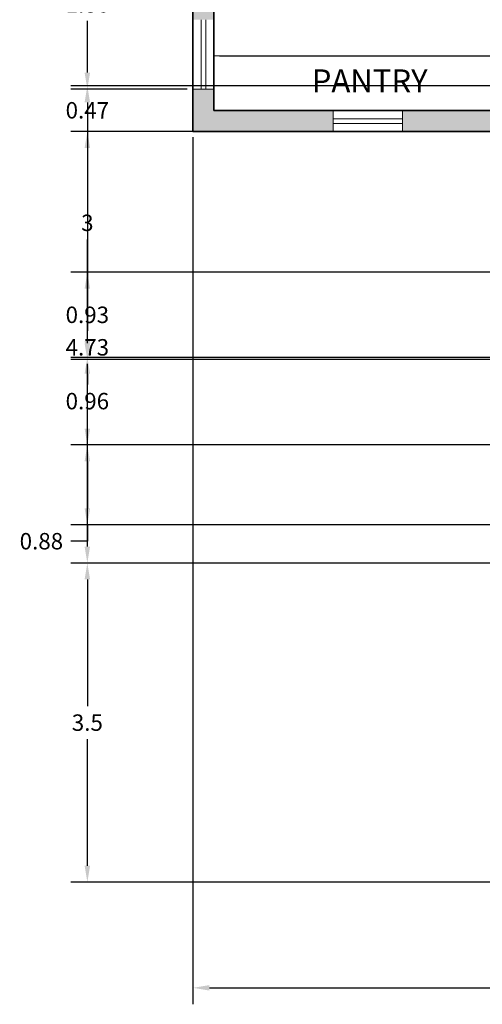
# Model space of a CAD drawing. Units: metres. Extents: x 4298.5 to 4325.2, y 2075 to 2095.8.
# Tile 1 of 35: x 4298.5 to 4303.6, y 2075 to 2085.8. Entities that reach past the tile are written whole.
import ezdxf

# ---------------------------------------------------------------- set-up
doc = ezdxf.new("R2010")
doc.units = ezdxf.units.M
for name, color, linetype, lineweight in [('A-ANNO-DIMS', 2, 'Continuous', 18), ('A-AREA-IDEN', 7, 'Continuous', 18), ('A-FLOR-CASE', 8, 'Continuous', 18), ('A-GLAZ', 4, 'Continuous', 18), ('A-WALL', 7, 'Continuous', 35), ('A-WALL-PATT', 252, 'Continuous', 13)]:
    doc.layers.add(name, color=color, linetype=linetype, lineweight=lineweight)
doc.styles.get("Standard").update_dxf_attribs({"font": 'arial.ttf'})
doc.dimstyles.get("Standard").update_dxf_attribs({"dimtxt": 0.18, "dimasz": 0.18, "dimexe": 0.18, "dimexo": 0.0625, "dimgap": 0.09, "dimtad": 0, "dimtih": 1, "dimtoh": 1, "dimdec": 4, "dimzin": 0, "dimdsep": 46, "dimtxsty": 'Standard', "dimcen": 0.09, "dimadec": 0, "dimazin": 0, "dimtfac": 1, "dimtdec": 4, "dimtofl": 0, "dimtmove": 0, "dimatfit": 3, "dimfxl": 1, "dimtolj": 1, "dimtzin": 0, "dimarcsym": 0})

# ---------------------------------------------------------------- blocks, each defined once
blk = doc.blocks.new('WIN-760-GLASS')
for p, q in [((0, 0.76), (0, 0)), ((0.05, 0.76), (0.05, 0))]:
    blk.add_line(p, q)
blk = doc.blocks.new('*D47')
at = {"layer": 'A-ANNO-DIMS', "color": 0, "lineweight": -2, "transparency": 16777216}
for p, q in [((4300.431, 2084.496), (4300.431, 2074.99)), ((4322.811, 2084.496), (4322.811, 2074.99)), ((4300.611, 2075.17), (4311.225, 2075.17)), ((4322.631, 2075.17), (4312.016, 2075.17))]:
    blk.add_line(p, q, dxfattribs=at)
at = {"layer": 'A-ANNO-DIMS', "color": 0, "transparency": 16777216}
for points in [[(4300.611, 2075.2), (4300.611, 2075.14), (4300.431, 2075.17)], [(4322.631, 2075.2), (4322.631, 2075.14), (4322.811, 2075.17)]]:
    blk.add_solid(points, dxfattribs=at)
at = {"layer": 'Defpoints', "color": 0, "transparency": 16777216}
for p in [(4300.431, 2084.558), (4322.811, 2084.558), (4322.811, 2075.17)]:
    blk.add_point(p, dxfattribs=at)
at = {"layer": 'A-ANNO-DIMS', "color": 0, "transparency": 16777216, "insert": (4311.621, 2075.17), "char_height": 0.18, "attachment_point": 5}
blk.add_mtext('\\A1;22.38', dxfattribs=at)
blk = doc.blocks.new('*D51')
at = {"layer": 'A-ANNO-DIMS', "color": 0, "lineweight": -2, "transparency": 16777216}
for p, q in [((4305.598, 2084.558), (4299.092, 2084.558)), ((4299.272, 2084.378), (4299.272, 2082.375)), ((4299.272, 2080.008), (4299.272, 2082.011)), ((4305.598, 2079.828), (4299.092, 2079.828))]:
    blk.add_line(p, q, dxfattribs=at)
at = {"layer": 'A-ANNO-DIMS', "color": 0, "transparency": 16777216}
for points in [[(4299.242, 2084.378), (4299.302, 2084.378), (4299.272, 2084.558)], [(4299.242, 2080.008), (4299.302, 2080.008), (4299.272, 2079.828)]]:
    blk.add_solid(points, dxfattribs=at)
at = {"layer": 'Defpoints', "color": 0, "transparency": 16777216}
for p in [(4305.661, 2084.558), (4299.272, 2079.828), (4305.661, 2079.828)]:
    blk.add_point(p, dxfattribs=at)
at = {"layer": 'A-ANNO-DIMS', "color": 0, "transparency": 16777216, "insert": (4299.272, 2082.193), "char_height": 0.18, "attachment_point": 5}
blk.add_mtext('\\A1;4.73', dxfattribs=at)
blk = doc.blocks.new('*D54')
at = {"layer": 'A-ANNO-DIMS', "color": 0, "lineweight": -2, "transparency": 16777216}
for p, q in [((4305.598, 2079.828), (4299.092, 2079.828)), ((4299.272, 2079.648), (4299.272, 2078.26)), ((4299.272, 2076.508), (4299.272, 2077.896)), ((4309.098, 2076.328), (4299.092, 2076.328))]:
    blk.add_line(p, q, dxfattribs=at)
at = {"layer": 'A-ANNO-DIMS', "color": 0, "transparency": 16777216}
for points in [[(4299.242, 2079.648), (4299.302, 2079.648), (4299.272, 2079.828)], [(4299.242, 2076.508), (4299.302, 2076.508), (4299.272, 2076.328)]]:
    blk.add_solid(points, dxfattribs=at)
at = {"layer": 'Defpoints', "color": 0, "transparency": 16777216}
for p in [(4305.661, 2079.828), (4299.272, 2076.328), (4309.161, 2076.328)]:
    blk.add_point(p, dxfattribs=at)
at = {"layer": 'A-ANNO-DIMS', "color": 0, "transparency": 16777216, "insert": (4299.272, 2078.078), "char_height": 0.18, "attachment_point": 5}
blk.add_mtext('\\A1;3.5', dxfattribs=at)
blk = doc.blocks.new('*D56')
at = {"layer": 'A-ANNO-DIMS', "color": 0, "lineweight": -2, "transparency": 16777216}
for p, q in [((4305.828, 2085.058), (4299.092, 2085.058)), ((4299.272, 2084.878), (4299.272, 2083.74)), ((4299.272, 2082.238), (4299.272, 2083.376)), ((4305.828, 2082.058), (4299.092, 2082.058))]:
    blk.add_line(p, q, dxfattribs=at)
at = {"layer": 'A-ANNO-DIMS', "color": 0, "transparency": 16777216}
for points in [[(4299.242, 2084.878), (4299.302, 2084.878), (4299.272, 2085.058)], [(4299.242, 2082.238), (4299.302, 2082.238), (4299.272, 2082.058)]]:
    blk.add_solid(points, dxfattribs=at)
at = {"layer": 'Defpoints', "color": 0, "transparency": 16777216}
for p in [(4299.272, 2085.058), (4305.891, 2085.058), (4305.891, 2082.058)]:
    blk.add_point(p, dxfattribs=at)
at = {"layer": 'A-ANNO-DIMS', "color": 0, "transparency": 16777216, "insert": (4299.272, 2083.558), "char_height": 0.18, "attachment_point": 5}
blk.add_mtext('\\A1;3', dxfattribs=at)
blk = doc.blocks.new('*D58')
at = {"layer": 'A-ANNO-DIMS', "color": 0, "lineweight": -2, "transparency": 16777216}
for p, q in [((4324.587, 2085.388), (4324.587, 2085.568)), ((4324.587, 2085.568), (4324.767, 2085.568)), ((4300.723, 2085.388), (4324.767, 2085.388)), ((4324.587, 2084.968), (4324.587, 2085.208)), ((4300.723, 2084.788), (4324.767, 2084.788))]:
    blk.add_line(p, q, dxfattribs=at)
at = {"layer": 'A-ANNO-DIMS', "color": 0, "transparency": 16777216}
for points in [[(4324.557, 2085.208), (4324.617, 2085.208), (4324.587, 2085.388)], [(4324.557, 2084.968), (4324.617, 2084.968), (4324.587, 2084.788)]]:
    blk.add_solid(points, dxfattribs=at)
at = {"layer": 'Defpoints', "color": 0, "transparency": 16777216}
for p in [(4300.661, 2085.388), (4324.587, 2085.388), (4300.661, 2084.788)]:
    blk.add_point(p, dxfattribs=at)
at = {"layer": 'A-ANNO-DIMS', "color": 0, "transparency": 16777216, "insert": (4325.021, 2085.568), "char_height": 0.18, "attachment_point": 5}
blk.add_mtext('\\A1;0.6', dxfattribs=at)
blk = doc.blocks.new('*D62')
at = {"layer": 'A-ANNO-DIMS', "color": 0, "lineweight": -2, "transparency": 16777216}
for p, q in [((4312.11, 2083.015), (4299.092, 2083.015)), ((4299.272, 2082.835), (4299.272, 2082.731)), ((4299.272, 2082.263), (4299.272, 2082.367)), ((4312.11, 2082.083), (4299.092, 2082.083))]:
    blk.add_line(p, q, dxfattribs=at)
at = {"layer": 'A-ANNO-DIMS', "color": 0, "transparency": 16777216}
for points in [[(4299.242, 2082.835), (4299.302, 2082.835), (4299.272, 2083.015)], [(4299.242, 2082.263), (4299.302, 2082.263), (4299.272, 2082.083)]]:
    blk.add_solid(points, dxfattribs=at)
at = {"layer": 'Defpoints', "color": 0, "transparency": 16777216}
for p in [(4312.172, 2083.015), (4299.272, 2082.083), (4312.172, 2082.083)]:
    blk.add_point(p, dxfattribs=at)
at = {"layer": 'A-ANNO-DIMS', "color": 0, "transparency": 16777216, "insert": (4299.272, 2082.549), "char_height": 0.18, "attachment_point": 5}
blk.add_mtext('\\A1;0.93', dxfattribs=at)
blk = doc.blocks.new('*D63')
at = {"layer": 'A-ANNO-DIMS', "color": 0, "lineweight": -2, "transparency": 16777216}
for p, q in [((4312.11, 2082.083), (4299.092, 2082.083)), ((4299.272, 2081.903), (4299.272, 2081.785)), ((4299.272, 2081.302), (4299.272, 2081.421)), ((4312.11, 2081.122), (4299.092, 2081.122))]:
    blk.add_line(p, q, dxfattribs=at)
at = {"layer": 'A-ANNO-DIMS', "color": 0, "transparency": 16777216}
for points in [[(4299.242, 2081.903), (4299.302, 2081.903), (4299.272, 2082.083)], [(4299.242, 2081.302), (4299.302, 2081.302), (4299.272, 2081.122)]]:
    blk.add_solid(points, dxfattribs=at)
at = {"layer": 'Defpoints', "color": 0, "transparency": 16777216}
for p in [(4312.172, 2082.083), (4299.272, 2081.122), (4312.172, 2081.122)]:
    blk.add_point(p, dxfattribs=at)
at = {"layer": 'A-ANNO-DIMS', "color": 0, "transparency": 16777216, "insert": (4299.272, 2081.603), "char_height": 0.18, "attachment_point": 5}
blk.add_mtext('\\A1;0.96', dxfattribs=at)
blk = doc.blocks.new('*D64')
at = {"layer": 'A-ANNO-DIMS', "color": 0, "lineweight": -2, "transparency": 16777216}
for p, q in [((4312.11, 2081.122), (4299.092, 2081.122)), ((4299.272, 2080.942), (4299.272, 2080.427)), ((4312.11, 2080.247), (4299.092, 2080.247)), ((4299.272, 2080.247), (4299.272, 2080.067)), ((4299.272, 2080.067), (4299.092, 2080.067))]:
    blk.add_line(p, q, dxfattribs=at)
at = {"layer": 'A-ANNO-DIMS', "color": 0, "transparency": 16777216}
for points in [[(4299.242, 2080.942), (4299.302, 2080.942), (4299.272, 2081.122)], [(4299.242, 2080.427), (4299.302, 2080.427), (4299.272, 2080.247)]]:
    blk.add_solid(points, dxfattribs=at)
at = {"layer": 'Defpoints', "color": 0, "transparency": 16777216}
for p in [(4312.172, 2081.122), (4299.272, 2080.247), (4312.172, 2080.247)]:
    blk.add_point(p, dxfattribs=at)
at = {"layer": 'A-ANNO-DIMS', "color": 0, "transparency": 16777216, "insert": (4298.768, 2080.067), "char_height": 0.18, "attachment_point": 5}
blk.add_mtext('\\A1;0.88', dxfattribs=at)
blk = doc.blocks.new('*D74')
at = {"layer": 'A-ANNO-DIMS', "color": 0, "lineweight": -2, "transparency": 16777216}
for p, q in [((4299.272077, 2085.20492), (4299.272077, 2085.38492)), ((4300.368077, 2085.02492), (4299.092077, 2085.02492)), ((4300.368077, 2084.558056), (4299.092077, 2084.558056)), ((4299.272077, 2084.378056), (4299.272077, 2084.198056))]:
    blk.add_line(p, q, dxfattribs=at)
at = {"layer": 'A-ANNO-DIMS', "color": 0, "transparency": 16777216}
for points in [[(4299.242077, 2085.20492), (4299.302077, 2085.20492), (4299.272077, 2085.02492)], [(4299.242077, 2084.378056), (4299.302077, 2084.378056), (4299.272077, 2084.558056)]]:
    blk.add_solid(points, dxfattribs=at)
at = {"layer": 'Defpoints', "color": 0, "transparency": 16777216}
for p in [(4299.272077, 2085.02492), (4300.430577, 2085.02492), (4300.430577, 2084.558056)]:
    blk.add_point(p, dxfattribs=at)
at = {"layer": 'A-ANNO-DIMS', "color": 0, "transparency": 16777216, "insert": (4299.272077, 2084.791488), "char_height": 0.18, "attachment_point": 5}
blk.add_mtext('\\A1;0.47', dxfattribs=at)
blk = doc.blocks.new('*D75')
at = {"layer": 'A-ANNO-DIMS', "color": 0, "lineweight": -2, "transparency": 16777216}
for p, q in [((4300.368, 2086.884), (4299.092, 2086.884)), ((4299.272, 2086.704), (4299.272, 2086.137)), ((4299.272, 2085.205), (4299.272, 2085.773)), ((4300.368, 2085.025), (4299.092, 2085.025))]:
    blk.add_line(p, q, dxfattribs=at)
at = {"layer": 'A-ANNO-DIMS', "color": 0, "transparency": 16777216}
for points in [[(4299.242, 2086.704), (4299.302, 2086.704), (4299.272, 2086.884)], [(4299.242, 2085.205), (4299.302, 2085.205), (4299.272, 2085.025)]]:
    blk.add_solid(points, dxfattribs=at)
at = {"layer": 'Defpoints', "color": 0, "transparency": 16777216}
for p in [(4299.272, 2086.884), (4300.431, 2086.884), (4300.431, 2085.025)]:
    blk.add_point(p, dxfattribs=at)
at = {"layer": 'A-ANNO-DIMS', "color": 0, "transparency": 16777216, "insert": (4299.272, 2085.955), "char_height": 0.18, "attachment_point": 5}
blk.add_mtext('\\A1;1.86', dxfattribs=at)

msp = doc.modelspace()

# ---------------------------------------------------------------- hatches: boundary and pattern name
at = {"layer": 'A-WALL-PATT'}
h = msp.add_hatch(color=256, dxfattribs=at)
h.dxf.hatch_style = 1
h.paths.add_polyline_path([(4308.7606, 2094.4781), (4308.1606, 2094.4781), (4307.4606, 2094.4781), (4307.4606, 2094.2481), (4308.2706, 2094.2481), (4308.2706, 2094.1281), (4308.3906, 2094.1281), (4308.3906, 2094.2481), (4308.7606, 2094.2481)])
h.paths.add_polyline_path([(4310.1206, 2094.4781), (4309.5206, 2094.4781), (4309.5206, 2094.2481), (4309.8906, 2094.2481), (4309.8906, 2092.2481), (4308.3906, 2092.2481), (4308.3906, 2093.4281), (4308.2706, 2093.4281), (4308.2706, 2092.0181), (4309.8906, 2092.0181), (4309.8906, 2087.0181), (4309.7706, 2087.0181), (4309.7706, 2086.7881), (4309.8906, 2086.7881), (4311.9406, 2086.7881), (4311.9406, 2087.0181), (4310.1206, 2087.0181), (4310.1206, 2089.0181), (4310.2406, 2089.0181), (4310.2406, 2089.1381), (4310.1206, 2089.1381), (4310.1206, 2092.0181), (4310.3078, 2092.0181), (4310.3078, 2092.2481), (4310.1206, 2092.2481)])
h.paths.add_polyline_path([(4311.7406, 2092.2481), (4311.0678, 2092.2481), (4311.0678, 2092.0181), (4311.7406, 2092.0181)], flags=17)
h.paths.add_polyline_path([(4313.1733, 2092.2481), (4312.5006, 2092.2481), (4312.5006, 2092.0181), (4313.1733, 2092.0181)])
h.paths.add_polyline_path([(4314.5378, 2092.2481), (4314.1206, 2092.2481), (4313.9333, 2092.2481), (4313.9333, 2092.0181), (4314.1206, 2092.0181), (4314.1206, 2087.0181), (4314.0006, 2087.0181), (4314.0006, 2086.7881), (4314.1206, 2086.7881), (4315.5718, 2086.7881), (4315.5718, 2087.0181), (4314.3506, 2087.0181), (4314.3506, 2092.0181), (4314.5378, 2092.0181)])
h.paths.add_polyline_path([(4315.9706, 2092.2481), (4315.2978, 2092.2481), (4315.2978, 2092.0181), (4315.9706, 2092.0181)])
h.paths.add_polyline_path([(4317.4033, 2092.2481), (4316.7306, 2092.2481), (4316.7306, 2092.0181), (4317.4033, 2092.0181)])
h.paths.add_polyline_path([(4318.9506, 2092.2481), (4318.3506, 2092.2481), (4318.1633, 2092.2481), (4318.1633, 2092.0181), (4318.3506, 2092.0181), (4318.3506, 2091.8981), (4318.5806, 2091.8981), (4318.5806, 2092.0181), (4318.9506, 2092.0181)])
h.paths.add_polyline_path([(4321.0106, 2092.2481), (4319.7106, 2092.2481), (4319.7106, 2092.0181), (4320.0806, 2092.0181), (4320.0806, 2090.0181), (4318.5806, 2090.0181), (4318.5806, 2091.1981), (4318.3506, 2091.1981), (4318.3506, 2090.0181), (4318.3506, 2087.0181), (4318.2306, 2087.0181), (4318.2306, 2086.7881), (4318.3506, 2086.7881), (4318.3506, 2086.3081), (4318.5806, 2086.3081), (4318.5806, 2089.7881), (4321.7806, 2089.7881), (4321.7806, 2090.0181), (4320.2006, 2090.0181), (4320.2006, 2092.0181), (4321.0106, 2092.0181)])
h.paths.add_polyline_path([(4322.8106, 2092.2481), (4321.7706, 2092.2481), (4321.7706, 2092.0181), (4322.5806, 2092.0181), (4322.5806, 2091.2831), (4322.8106, 2091.2831)])
h.paths.add_polyline_path([(4322.8106, 2090.5231), (4322.5806, 2090.5231), (4322.5806, 2089.7881), (4322.5806, 2089.5254), (4322.8106, 2089.5254), (4322.8106, 2090.0181)])
h.paths.add_polyline_path([(4322.8106, 2088.7654), (4322.5806, 2088.7654), (4322.5806, 2087.6681), (4322.8106, 2087.6681)])
h.paths.add_polyline_path([(4322.8106, 2086.9081), (4322.5806, 2086.9081), (4322.5806, 2085.8107), (4322.8106, 2085.8107)])
h.paths.add_polyline_path([(4322.8106, 2085.0507), (4322.5806, 2085.0507), (4322.5806, 2084.7881), (4318.5806, 2084.7881), (4318.5806, 2085.0581), (4318.5806, 2085.4081), (4318.3506, 2085.4081), (4318.3506, 2084.5581), (4318.3506, 2080.8581), (4318.4706, 2080.8581), (4318.4706, 2082.3281), (4319.2606, 2082.3281), (4319.2606, 2082.5581), (4318.5806, 2082.5581), (4318.5806, 2084.5581), (4320.0806, 2084.5581), (4320.0806, 2083.9381), (4320.3106, 2083.9381), (4320.3106, 2084.5581), (4322.8106, 2084.5581)])
h.paths.add_polyline_path([(4320.3106, 2083.1781), (4320.0806, 2083.1781), (4320.0806, 2082.5581), (4319.9606, 2082.5581), (4319.9606, 2082.3281), (4320.0806, 2082.3281), (4320.0806, 2081.5731), (4320.3106, 2081.5731)], flags=17)
h.paths.add_polyline_path([(4320.3106, 2080.8131), (4320.0806, 2080.8131), (4320.0806, 2080.0581), (4318.4286, 2080.0581), (4318.4286, 2079.8281), (4320.3106, 2079.8281)])
h.paths.add_polyline_path([(4317.3506, 2085.2881), (4316.5718, 2085.2881), (4316.5718, 2085.0581), (4317.3506, 2085.0581)])
h.paths.add_polyline_path([(4315.5718, 2085.2881), (4314.8434, 2085.2881), (4314.8434, 2085.0581), (4315.5718, 2085.0581)])
h.paths.add_polyline_path([(4313.8434, 2085.2881), (4312.9406, 2085.2881), (4312.9406, 2085.0581), (4313.8434, 2085.0581)])
h.paths.add_polyline_path([(4311.9406, 2085.2881), (4311.4406, 2085.2881), (4311.4406, 2085.0581), (4311.9406, 2085.0581)])
h.paths.add_polyline_path([(4317.3306, 2087.0181), (4316.5718, 2087.0181), (4316.5718, 2086.7881), (4317.3306, 2086.7881)])
h.paths.add_polyline_path([(4313.1006, 2089.1381), (4311.1406, 2089.1381), (4311.1406, 2089.0181), (4312.9806, 2089.0181), (4312.9806, 2087.0181), (4312.9406, 2087.0181), (4312.9406, 2086.7881), (4313.1006, 2086.7881), (4313.1006, 2087.0181)])
h.paths.add_polyline_path([(4307.5515, 2087.0181), (4305.8906, 2087.0181), (4305.8906, 2092.2481), (4305.8906, 2094.2481), (4306.7006, 2094.2481), (4306.7006, 2094.4781), (4305.6606, 2094.4781), (4305.6606, 2092.2481), (4305.2906, 2092.2481), (4305.2906, 2092.0181), (4305.6606, 2092.0181), (4305.6606, 2090.0181), (4304.1606, 2090.0181), (4304.1606, 2091.1981), (4304.0406, 2091.1981), (4304.0406, 2089.9081), (4301.5606, 2089.9081), (4301.5606, 2089.7881), (4304.0406, 2089.7881), (4305.6606, 2089.7881), (4305.6606, 2086.6381), (4305.8906, 2086.6381), (4305.8906, 2086.7881), (4307.5515, 2086.7881)])
h.paths.add_polyline_path([(4307.5515, 2085.2881), (4305.8906, 2085.2881), (4305.8906, 2085.4381), (4305.6606, 2085.4381), (4305.6606, 2084.7881), (4305.2906, 2084.7881), (4305.2906, 2084.5581), (4305.6606, 2084.5581), (4305.6606, 2084.02), (4305.8906, 2084.02), (4305.8906, 2084.5581), (4305.8906, 2085.0581), (4307.5515, 2085.0581)])
h.paths.add_polyline_path([(4310.2406, 2085.2881), (4308.5515, 2085.2881), (4308.5515, 2085.0581), (4310.2406, 2085.0581)])
h.paths.add_polyline_path([(4317.4286, 2080.0581), (4316.5718, 2080.0581), (4316.5718, 2079.8281), (4317.4286, 2079.8281)])
h.paths.add_polyline_path([(4315.5718, 2080.0581), (4314.8434, 2080.0581), (4314.8434, 2079.8281), (4315.5718, 2079.8281)])
h.paths.add_polyline_path([(4313.8434, 2080.0581), (4312.9406, 2080.0581), (4312.9406, 2079.8281), (4313.8434, 2079.8281)])
h.paths.add_polyline_path([(4311.9406, 2080.0581), (4311.4406, 2080.0581), (4311.4406, 2079.8281), (4311.9406, 2079.8281)])
h.paths.add_polyline_path([(4310.2406, 2080.0581), (4310.1206, 2080.0581), (4310.1206, 2084.0381), (4309.8906, 2084.0381), (4309.8906, 2080.0581), (4309.1606, 2080.0581), (4309.1606, 2079.8281), (4310.2406, 2079.8281)])
h.paths.add_polyline_path([(4308.1606, 2080.0581), (4307.5106, 2080.0581), (4307.5106, 2080.1781), (4307.3906, 2080.1781), (4307.3906, 2080.0581), (4305.8906, 2080.0581), (4305.8906, 2080.567), (4305.6606, 2080.567), (4305.6606, 2079.8281), (4308.1606, 2079.8281)])
h.paths.add_polyline_path([(4307.5106, 2081.9381), (4309.0906, 2081.9381), (4309.0906, 2082.0581), (4305.8906, 2082.0581), (4305.8906, 2083.26), (4305.6606, 2083.26), (4305.6606, 2081.327), (4305.8906, 2081.327), (4305.8906, 2081.9381), (4307.3906, 2081.9381), (4307.3906, 2080.8781), (4307.5106, 2080.8781)])
h.paths.add_polyline_path([(4304.5306, 2084.7881), (4302.7306, 2084.7881), (4302.7306, 2084.5581), (4304.5306, 2084.5581)])
h.paths.add_polyline_path([(4301.9706, 2084.7881), (4300.6606, 2084.7881), (4300.6606, 2085.0249), (4300.4306, 2085.0249), (4300.4306, 2084.5581), (4301.9706, 2084.5581)])
h.paths.add_polyline_path([(4300.6606, 2086.8843), (4300.4306, 2086.8843), (4300.4306, 2085.7849), (4300.6606, 2085.7849)])
h.paths.add_polyline_path([(4300.6606, 2089.1618), (4300.4306, 2089.1618), (4300.4306, 2087.6443), (4300.6606, 2087.6443)])
h.paths.add_polyline_path([(4300.6606, 2091.0212), (4300.4306, 2091.0212), (4300.4306, 2089.9218), (4300.6606, 2089.9218)])
h.paths.add_polyline_path([(4300.6606, 2092.0181), (4301.9706, 2092.0181), (4301.9706, 2092.2481), (4300.4306, 2092.2481), (4300.4306, 2091.7812), (4300.6606, 2091.7812)])
h.paths.add_polyline_path([(4304.5306, 2092.2481), (4302.7306, 2092.2481), (4302.7306, 2092.0181), (4304.0406, 2092.0181), (4304.0406, 2091.8981), (4304.1606, 2091.8981), (4304.1606, 2092.0181), (4304.5306, 2092.0181)], flags=17)

# ---------------------------------------------------------------- linework, layer by layer
at = {"layer": 'A-FLOR-CASE'}
msp.add_line((4305.6606, 2085.3881), (4300.6606, 2085.3881), dxfattribs=at)
at = {"layer": 'A-GLAZ'}
for p, q in [((4300.6606, 2085.0249), (4300.4306, 2085.0249)), ((4301.9706, 2084.5581), (4301.9706, 2084.7881)), ((4302.7306, 2084.5581), (4302.7306, 2084.7881))]:
    msp.add_line(p, q, dxfattribs=at)
at = {"layer": 'A-WALL'}
for p, q in [((4300.4306, 2084.5581), (4300.4306, 2092.2481)), ((4300.6606, 2084.7881), (4300.6606, 2089.7881)), ((4305.6606, 2084.7881), (4300.6606, 2084.7881)), ((4305.6606, 2084.5581), (4300.4306, 2084.5581))]:
    msp.add_line(p, q, dxfattribs=at)

# ---------------------------------------------------------------- block references
at = {"layer": 'A-GLAZ'}
msp.add_blockref('WIN-760-GLASS', (4300.5206, 2085.0249), dxfattribs=at)
at = {"layer": 'A-GLAZ', "rotation": 269.9999999999362}
msp.add_blockref('WIN-760-GLASS', (4301.9706, 2084.6981), dxfattribs=at)

# ---------------------------------------------------------------- texts
at = {"layer": 'A-AREA-IDEN', "insert": (4301.734, 2085.2402), "char_height": 0.25, "attachment_point": 1}
msp.add_mtext_dynamic_manual_height_columns('PANTRY', width=2.22034, gutter_width=12.5, heights=[0], dxfattribs=at)

# ---------------------------------------------------------------- dimensions: what is measured, and where the dimension line sits
at = {"layer": 'A-ANNO-DIMS'}
for base, p1, p2, override, picture, middle in [((4299.2721, 2086.8843), (4300.4306, 2085.0249), (4300.4306, 2086.8843), {"dimdec": 2, "dimlfac": 1, "dimrnd": 0, "dimzin": 0, "dimdsep": 46, "dimlunit": 2}, '*D75', (4299.2721, 2085.9546)), ((4324.5871, 2085.3881), (4300.6606, 2084.7881), (4300.6606, 2085.3881), {"dimdec": 1, "dimlfac": 1, "dimrnd": 0, "dimzin": 0, "dimdsep": 46, "dimlunit": 2}, '*D58', (4325.0209, 2085.5681)), ((4299.2721, 2085.0249), (4300.4306, 2084.5581), (4300.4306, 2085.0249), {"dimdec": 2, "dimlfac": 1, "dimrnd": 0, "dimzin": 0, "dimdsep": 46, "dimlunit": 2}, '*D74', (4299.2721, 2084.7915)), ((4299.2721, 2085.0581), (4305.8906, 2082.0581), (4305.8906, 2085.0581), {"dimdec": 0, "dimlfac": 1, "dimrnd": 0, "dimzin": 0, "dimdsep": 46, "dimlunit": 2}, '*D56', (4299.2721, 2083.5581)), ((4299.2721, 2079.8281), (4305.6606, 2084.5581), (4305.6606, 2079.8281), {"dimdec": 2, "dimlfac": 1, "dimrnd": 0, "dimzin": 0, "dimdsep": 46, "dimlunit": 2}, '*D51', (4299.2721, 2082.1931)), ((4299.2721, 2082.0835), (4312.1722, 2083.0153), (4312.1722, 2082.0835), {"dimdec": 2, "dimlfac": 1, "dimrnd": 0, "dimzin": 0, "dimdsep": 46, "dimlunit": 2}, '*D62', (4299.2721, 2082.5494)), ((4299.2721, 2081.1221), (4312.1722, 2082.0835), (4312.1722, 2081.1221), {"dimdec": 2, "dimlfac": 1, "dimrnd": 0, "dimzin": 0, "dimdsep": 46, "dimlunit": 2}, '*D63', (4299.2721, 2081.6028)), ((4299.2721, 2080.247), (4312.1722, 2081.1221), (4312.1722, 2080.247), {"dimdec": 2, "dimlfac": 1, "dimrnd": 0, "dimzin": 0, "dimdsep": 46, "dimlunit": 2}, '*D64', (4298.7681, 2080.067)), ((4299.2721, 2076.3281), (4305.6606, 2079.8281), (4309.1606, 2076.3281), {"dimdec": 1, "dimlfac": 1, "dimrnd": 0, "dimzin": 0, "dimdsep": 46, "dimlunit": 2}, '*D54', (4299.2721, 2078.0781))]:
    dim = msp.add_linear_dim(base=base, p1=p1, p2=p2, angle=90, dimstyle='Standard', override=override, dxfattribs=at)
    dim.commit()
    dim.dimension.update_dxf_attribs({"geometry": picture, "text_midpoint": middle})
dim = msp.add_linear_dim(base=(4322.8106, 2075.1696), p1=(4300.4306, 2084.5581), p2=(4322.8106, 2084.5581), dimstyle='Standard', override={"dimdec": 2, "dimlfac": 1, "dimrnd": 0, "dimzin": 0, "dimdsep": 46, "dimlunit": 2}, dxfattribs=at)
dim.commit()
dim.dimension.update_dxf_attribs({"geometry": '*D47', "text_midpoint": (4311.6206, 2075.1696)})

doc.saveas('drawing.dxf')
